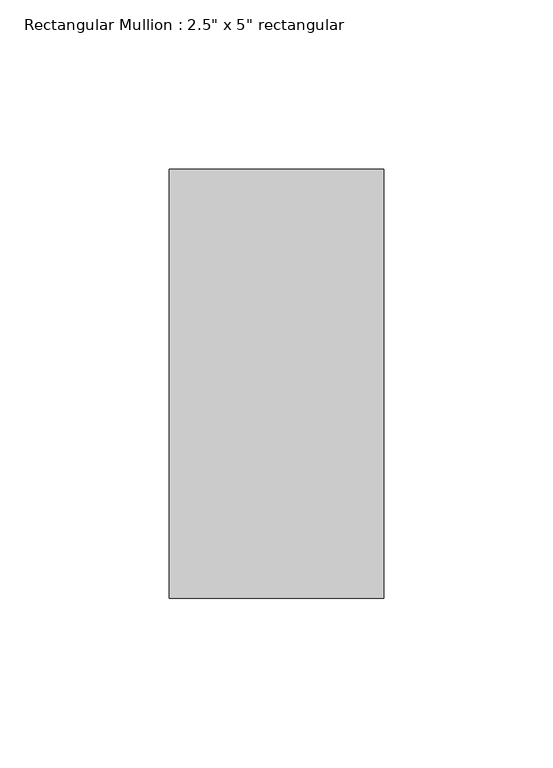
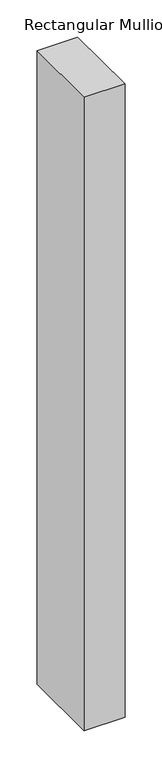
"""IFC4 building model written with IfcOpenShell, lengths in millimetres: member geometry."""

from ifc_helpers import new_model, si_unit, frame, origin, place, context, project, spatial, polyline, outline, extrude, source, transform, mapped, element, save


def member_8d8fe108(model_context):
    return source(origin(), model_context, "Body", "SweptSolid", [
        extrude(outline(polyline([(0.0, 63.5), (0.0, -63.5), (-63.5, -63.5), (-63.5, 63.5), (0.0, 63.5)])), frame((0.0, 0.0, -1041.4), z_axis=(0.0, 0.0, 1.0), x_axis=(1.0, 0.0, 0.0)), (0.0, 0.0, 1.0), 1041.4),
    ])


if __name__ == "__main__":
    model = new_model("IFC4")
    model_context = context("Model", 3, world=origin())
    ifc_project = project(units=[si_unit("LENGTHUNIT", "METRE", prefix="MILLI")], contexts=[model_context])
    site = spatial("IfcSite", under=ifc_project)
    building = spatial("IfcBuilding", under=site)
    placement = place(None, origin())
    member_shape = member_8d8fe108(model_context)
    element("IfcMember", 1, ObjectType="Rectangular Mullion : 2.5\" x 5\" rectangular", at=placement, inside=building, context=model_context, shape_type="MappedRepresentation", body=[
        mapped(member_shape, transform((0.0, 0.0, 0.0), x_axis=(1.0, 0.0, 0.0), y_axis=(0.0, 1.0, 0.0), z_axis=(0.0, 0.0, 1.0))),
    ])
    save(model, "model.ifc")

# Revit data of these elements
# Type "Rectangular Mullion : 2.5\" x 5\" rectangular"
#   built-in parameter 1007304 = 0.416667 (stored number, unit not read)
#   built-in parameter 1007301 = 0.104167 (stored number, unit not read)
#   built-in parameter 1007300 = 0.104167 (stored number, unit not read)
# Element 1 (IfcMember, "Rectangular Mullion : 2.5\" x 5\" rectangular")
#   Materials on its faces: "Aluminum"
# Materials
#   "Aluminum": class "Metal", colour RGB 247 247 247, transparency 0, Description = "Aluminum 6061", Cost = 0
